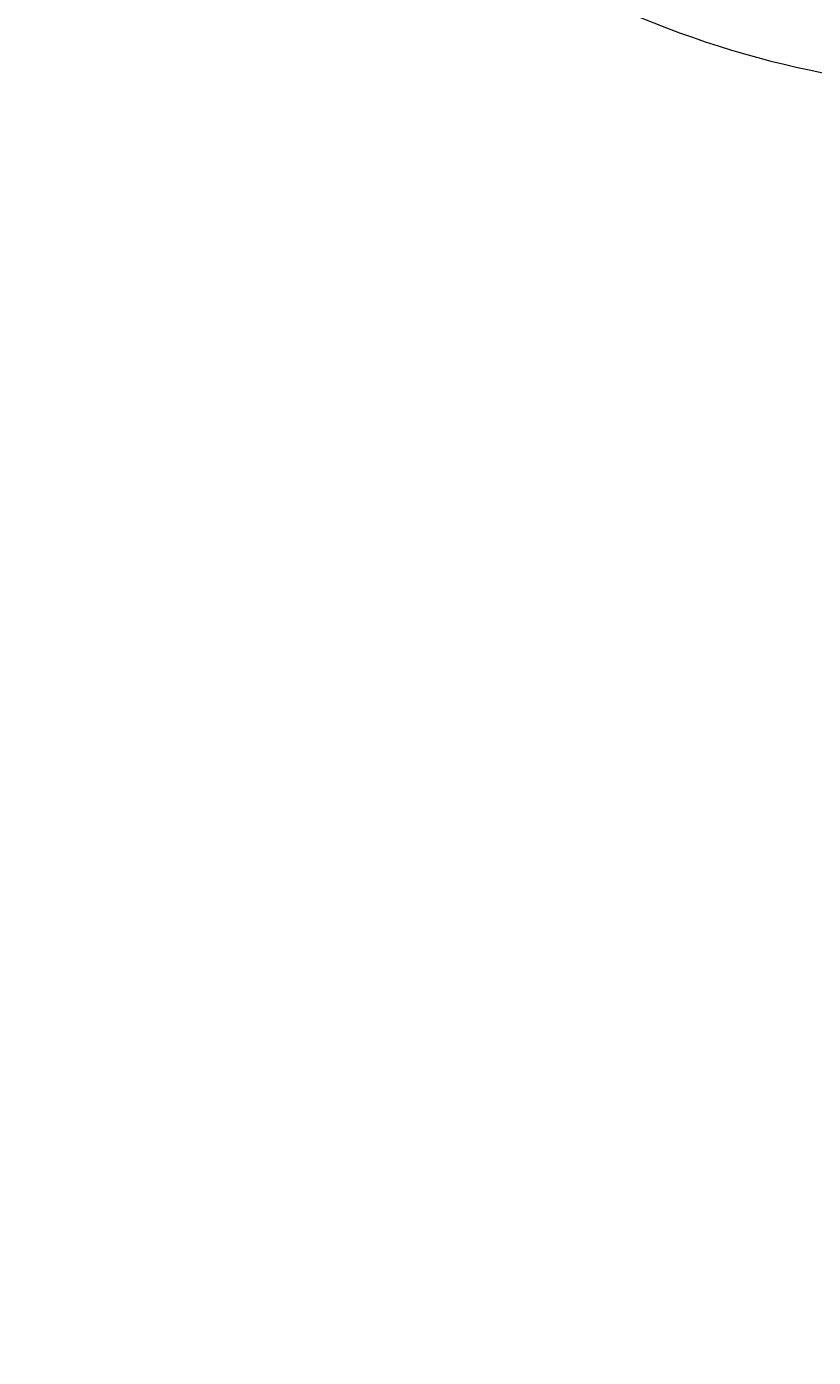
# Model space of a CAD drawing. Units: inches. Extents: x 1962 to 2771, y 1245 to 2660.
# Tile 56 of 114: x 2200 to 2224, y 2105 to 2145. Entities that reach past the tile are written whole.
import ezdxf

# ---------------------------------------------------------------- set-up
doc = ezdxf.new("R2010")
doc.units = ezdxf.units.IN
doc.layers.add('A-ANNO-DIMS', color=2, linetype='Continuous', lineweight=18)
doc.layers.add('A-DOOR', color=3, linetype='Continuous', lineweight=18)
doc.styles.get("Standard").update_dxf_attribs({"font": 'arial.ttf'})
doc.dimstyles.get("Standard").update_dxf_attribs({"dimtxt": 0.18, "dimasz": 0.18, "dimexe": 0.18, "dimexo": 0.0625, "dimgap": 0.09, "dimtad": 0, "dimtih": 1, "dimtoh": 1, "dimdec": 4, "dimzin": 0, "dimdsep": 46, "dimtxsty": 'Standard', "dimcen": 0.09, "dimadec": 0, "dimazin": 0, "dimtfac": 1, "dimtdec": 4, "dimtofl": 0, "dimtmove": 0, "dimatfit": 3, "dimfxl": 1, "dimtolj": 1, "dimtzin": 0, "dimarcsym": 0})

# ---------------------------------------------------------------- blocks, each defined once
blk = doc.blocks.new('*D40')
at = {"layer": 'A-ANNO-DIMS', "color": 0, "lineweight": -2, "transparency": 16777216}
for p, q in [((2072.02, 2033.906), (2072.02, 2583.474)), ((2072.2, 2583.294), (2366.02, 2583.294)), ((2660.627, 2583.294), (2366.808, 2583.294)), ((2660.807, 2524.406), (2660.807, 2583.474))]:
    blk.add_line(p, q, dxfattribs=at)
at = {"layer": 'A-ANNO-DIMS', "color": 0, "transparency": 16777216}
for points in [[(2072.2, 2583.324), (2072.2, 2583.264), (2072.02, 2583.294)], [(2660.627, 2583.324), (2660.627, 2583.264), (2660.807, 2583.294)]]:
    blk.add_solid(points, dxfattribs=at)
at = {"layer": 'Defpoints', "color": 0, "transparency": 16777216}
for p in [(2660.807, 2583.294), (2660.807, 2524.344), (2072.02, 2033.844)]:
    blk.add_point(p, dxfattribs=at)
at = {"layer": 'A-ANNO-DIMS', "color": 0, "transparency": 16777216, "insert": (2366.414, 2583.294), "char_height": 0.18, "attachment_point": 5}
blk.add_mtext('\\A1;588.8', dxfattribs=at)

msp = doc.modelspace()

# ---------------------------------------------------------------- linework, layer by layer
at = {"layer": 'A-DOOR'}
msp.add_arc((2229.2838, 2171.1428), 28.2264, 180, 286.41252, dxfattribs=at)

# ---------------------------------------------------------------- dimensions: what is measured, and where the dimension line sits
at = {"layer": 'A-ANNO-DIMS'}
dim = msp.add_linear_dim(base=(2660.8074, 2583.2937), p1=(2072.0204, 2033.8437), p2=(2660.8074, 2524.3437), dimstyle='Standard', override={"dimdec": 1, "dimlfac": 1, "dimrnd": 0, "dimzin": 0, "dimdsep": 46, "dimlunit": 2}, dxfattribs=at)
dim.commit()
dim.dimension.update_dxf_attribs({"geometry": '*D40', "text_midpoint": (2366.4139, 2583.2937)})

doc.saveas('drawing.dxf')
